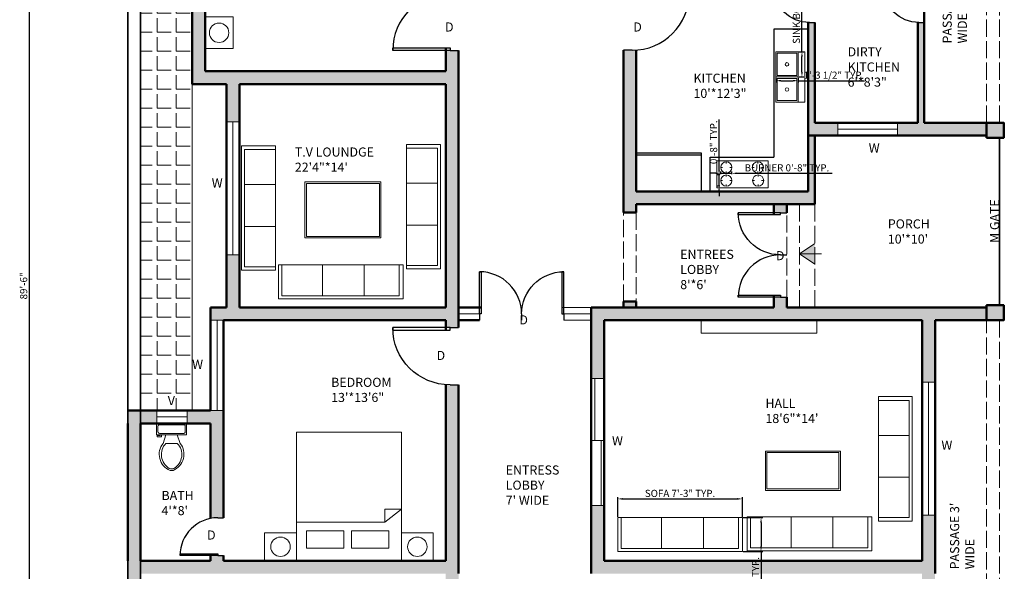
# Model space of a CAD drawing. Units: inches. Extents: x 554 to 1300, y 1707 to 2873.
# Tile 2 of 3: x 554 to 1242, y 2105 to 2490. Entities that reach past the tile are written whole.
import ezdxf

# ---------------------------------------------------------------- set-up
doc = ezdxf.new("R2010")
doc.units = ezdxf.units.IN
doc.linetypes.add('ACAD_ISO02W100', pattern=[15, 12, -3])
for name, color, linetype, lineweight in [('A-ANNO-DIMS', 145, 'Continuous', 18), ('A-ANNO-PATT', 7, 'Continuous', 13), ('A-ANNO-SYMB', 7, 'Continuous', 18), ('A-AREA-IDEN', 145, 'Continuous', 25), ('A-CASE', 8, 'Continuous', 25), ('A-EQPM', 9, 'Continuous', 18), ('A-FLOR-FIXT', 9, 'Continuous', 18), ('A-FLOR-OVHD', 8, 'ACAD_ISO02W100', 18), ('A-WALL-OVHD', 30, 'ACAD_ISO02W100', 18), ('A-WALL-PATT', 30, 'Continuous', 13), ('C-PROP', 30, 'Continuous', 35), ('C-PROP-OVHD', 30, 'ACAD_ISO02W100', 18), ('C-PVMT', 8, 'Continuous', 18), ('C-PVMT-PATT', 116, 'Continuous', 13), ('COLUMN', 30, 'Continuous', 50), ('DOOR', 52, 'Continuous', 25), ('FUR', 210, 'Continuous', 18), ('TEXT', 145, 'Continuous', 18), ('WALL', 30, 'Continuous', 50), ('WIND', 70, 'Continuous', 18)]:
    doc.layers.add(name, color=color, linetype=linetype, lineweight=lineweight)
doc.styles.get("Standard").update_dxf_attribs({"font": 'arial.ttf'})
doc.dimstyles.new('ISO-25', dxfattribs={"dimtxt": 5, "dimasz": 3.5, "dimexe": 1.25, "dimexo": 0.625, "dimtad": 1, "dimdec": 0, "dimlunit": 4, "dimtxsty": 'Standard', "dimcen": 2.5, "dimadec": 0, "dimazin": 0, "dimtfac": 1, "dimtdec": 0, "dimtmove": 0, "dimatfit": 3, "dimfxl": 1, "dimarcsym": 0})

# ---------------------------------------------------------------- blocks, each defined once
blk = doc.blocks.new('*U2')
for p, q in [((0, 0), (0, -6)), ((40, 0), (40, -6))]:
    blk.add_line(p, q)
blk.add_lwpolyline([(0, 0), (0, 40), (1.75, 40), (1.75, 0)], close=True)
blk.add_arc((0, 0), 40, 0, 90)
blk = doc.blocks.new('*U4')
for p, q in [((9.5, -6), (9.5, -2)), ((-10, -8.5), (-8, -8.5)), ((-10, -9.5), (-10, -8.5)), ((-7, -9.5), (-10, -9.5)), ((-8, -8.5), (-8, -8)), ((-7, -8), (-7, -9.5)), ((-4, -8), (-6, -14)), ((4, -8), (6, -14)), ((4, -14), (-4, -14))]:
    blk.add_line(p, q)
blk.add_lwpolyline([(10.5, -8), (10.5, 0), (-10.5, 0), (-10.5, -8)], close=True)
for points in [[(-9.5, -2), (-9.5, -6)], [(8.5, -1), (-8.5, -1)], [(-8.5, -7), (8.5, -7)]]:
    blk.add_lwpolyline(points)
for centre, radius, start, end in [((-8.62, -1.88), 0.884, 81.8699, 188.1301), ((-8.62, -6.12), 0.884, 171.8699, 278.1301), ((8.62, -1.88), 0.884, 351.8699, 98.1301), ((8.62, -6.12), 0.884, 261.8699, 8.1301), ((3.52, -21.58), 12.17, 141.46911, 247.97143), ((4.2, -21.82), 11.33, 136.36773, 238.94682), ((-3.52, -21.58), 12.17, 292.02843, 38.53071), ((-4.2, -21.82), 11.33, 301.05301, 43.63209), ((0, -27.88), 4, 245.73182, 294.26817), ((0, -29), 4, 254.86053, 285.13947)]:
    blk.add_arc(centre, radius, start, end)
blk = doc.blocks.new('*D8')
at = {"layer": 'A-ANNO-DIMS', "color": 0, "lineweight": -2, "transparency": 16777216}
for p, q in [((629.06, 2841.48), (559.64, 2841.48)), ((560.89, 2837.98), (560.89, 1770.98)), ((629.06, 1767.48), (559.64, 1767.48))]:
    blk.add_line(p, q, dxfattribs=at)
at = {"layer": 'A-ANNO-DIMS', "color": 0, "lineweight": 100, "transparency": 16777216}
for points in [[(560.3, 2837.98), (561.47, 2837.98), (560.89, 2841.48)], [(560.3, 1770.98), (561.47, 1770.98), (560.89, 1767.48)]]:
    blk.add_solid(points, dxfattribs=at)
at = {"layer": 'Defpoints', "color": 0, "lineweight": 100, "transparency": 16777216}
for p in [(629.68, 2841.48), (560.89, 1767.48), (629.68, 1767.48)]:
    blk.add_point(p, dxfattribs=at)
at = {"layer": 'A-ANNO-DIMS', "color": 0, "transparency": 16777216, "insert": (557.71, 2304.48), "char_height": 5, "attachment_point": 5, "rotation": 90}
blk.add_mtext('89\'-6"', dxfattribs=at)
blk = doc.blocks.new('SOFA-3SEAT')
for p, q in [((0, 84.31), (0, 87)), ((0, 87), (23.69, 87)), ((23.69, 87), (23.69, 0)), ((0, 59.83), (21.61, 59.83)), ((0, 30.66), (21.61, 30.66)), ((0, 0), (0, 5.47)), ((23.69, 0), (0, 0))]:
    blk.add_line(p, q)
blk.add_lwpolyline([(21.61, 84.31), (0, 84.31), (0, 2.38), (21.61, 2.38)], close=True)
blk = doc.blocks.new('NIGHTSTAND')
blk.add_lwpolyline([(22.14, 19.58), (0, 19.58), (0, 0), (22.14, 0)], close=True)
blk.add_circle((11.07, 9.79), 6.79)
blk = doc.blocks.new('TABLE-COFFEE')
for points in [[(52.29, 0), (0, 0), (0, 27.46), (52.29, 27.46)], [(51.29, 1), (1, 1), (1, 26.46), (51.29, 26.46)]]:
    blk.add_lwpolyline(points, close=True)
blk = doc.blocks.new('COOKTOP-BURNER')
for p, q in [((3.89, 7.77), (3.89, 6.66)), ((0, 3.89), (1.24, 3.89)), ((3.89, 0), (3.89, 1.05)), ((7.77, 3.89), (6.32, 3.89))]:
    blk.add_line(p, q)
blk.add_circle((3.89, 3.89), 3.89)
blk = doc.blocks.new('SINK-BOWL-RECT')
for points in [[(0, 0), (15.58, 0), (15.58, 17.58), (0, 17.58)], [(1, 1), (14.58, 1), (14.58, 16.58), (1, 16.58)]]:
    blk.add_lwpolyline(points, close=True)
blk.add_circle((7.79, 8.79), 1.21)
blk = doc.blocks.new('*D16')
at = {"layer": 'A-ANNO-DIMS', "color": 0, "lineweight": -2, "transparency": 16777216}
for p, q in [((971.7, 2143.27), (971.7, 2156.95)), ((975.2, 2155.7), (1055.2, 2155.7)), ((1058.7, 2143.27), (1058.7, 2156.95))]:
    blk.add_line(p, q, dxfattribs=at)
at = {"layer": 'A-ANNO-DIMS', "color": 0, "lineweight": 100, "transparency": 16777216}
for points in [[(975.2, 2156.28), (975.2, 2155.11), (971.7, 2155.7)], [(1055.2, 2156.28), (1055.2, 2155.11), (1058.7, 2155.7)]]:
    blk.add_solid(points, dxfattribs=at)
at = {"layer": 'Defpoints', "color": 0, "lineweight": 100, "transparency": 16777216}
for p in [(1058.7, 2155.7), (971.7, 2142.65), (1058.7, 2142.65)]:
    blk.add_point(p, dxfattribs=at)
at = {"layer": 'A-ANNO-DIMS', "color": 0, "transparency": 16777216, "insert": (1015.2, 2158.91), "char_height": 5, "attachment_point": 5}
blk.add_mtext('SOFA 7\'-3" TYP.', dxfattribs=at)
blk = doc.blocks.new('*D17')
at = {"layer": 'A-ANNO-DIMS', "color": 0, "lineweight": -2, "transparency": 16777216}
for p, q in [((1059.32, 2142.65), (1073, 2142.65)), ((1071.75, 2139.15), (1071.75, 2122.46)), ((1059.32, 2118.96), (1073, 2118.96)), ((1071.75, 2118.96), (1071.75, 2068.67))]:
    blk.add_line(p, q, dxfattribs=at)
at = {"layer": 'A-ANNO-DIMS', "color": 0, "lineweight": 100, "transparency": 16777216}
for points in [[(1071.16, 2139.15), (1072.33, 2139.15), (1071.75, 2142.65)], [(1071.16, 2122.46), (1072.33, 2122.46), (1071.75, 2118.96)]]:
    blk.add_solid(points, dxfattribs=at)
at = {"layer": 'Defpoints', "color": 0, "lineweight": 100, "transparency": 16777216}
for p in [(1058.7, 2142.65), (1058.7, 2118.96), (1071.75, 2118.96)]:
    blk.add_point(p, dxfattribs=at)
at = {"layer": 'A-ANNO-DIMS', "color": 0, "transparency": 16777216, "insert": (1068.54, 2092.06), "char_height": 5, "attachment_point": 5, "rotation": 90}
blk.add_mtext('1\'-11 1/2" TYP.', dxfattribs=at)
blk = doc.blocks.new('*D20')
at = {"layer": 'A-ANNO-DIMS', "color": 0, "lineweight": -2, "transparency": 16777216}
for p, q in [((1040.11, 2383.13), (1036.61, 2383.13)), ((1043.61, 2382.59), (1043.61, 2384.38)), ((1043.61, 2383.13), (1051.38, 2383.13)), ((1051.38, 2382.59), (1051.38, 2384.38)), ((1054.88, 2383.13), (1121.32, 2383.13))]:
    blk.add_line(p, q, dxfattribs=at)
at = {"layer": 'A-ANNO-DIMS', "color": 0, "lineweight": 100, "transparency": 16777216}
for points in [[(1040.11, 2383.71), (1040.11, 2382.54), (1043.61, 2383.13)], [(1054.88, 2383.71), (1054.88, 2382.54), (1051.38, 2383.13)]]:
    blk.add_solid(points, dxfattribs=at)
at = {"layer": 'Defpoints', "color": 0, "lineweight": 100, "transparency": 16777216}
for p in [(1043.61, 2381.96), (1051.38, 2383.13), (1051.38, 2381.96)]:
    blk.add_point(p, dxfattribs=at)
at = {"layer": 'A-ANNO-DIMS', "color": 0, "transparency": 16777216, "insert": (1089.85, 2386.31), "char_height": 5, "attachment_point": 5}
blk.add_mtext('BURNER 0\'-8" TYP.', dxfattribs=at)
blk = doc.blocks.new('*D21')
at = {"layer": 'A-ANNO-DIMS', "color": 0, "lineweight": -2, "transparency": 16777216}
for p, q in [((1042.44, 2385.46), (1042.44, 2420.69)), ((1042.98, 2381.96), (1041.19, 2381.96)), ((1042.44, 2374.19), (1042.44, 2381.96)), ((1042.98, 2374.19), (1041.19, 2374.19)), ((1042.44, 2370.69), (1042.44, 2367.19))]:
    blk.add_line(p, q, dxfattribs=at)
at = {"layer": 'A-ANNO-DIMS', "color": 0, "lineweight": 100, "transparency": 16777216}
for points in [[(1041.86, 2385.46), (1043.02, 2385.46), (1042.44, 2381.96)], [(1041.86, 2370.69), (1043.02, 2370.69), (1042.44, 2374.19)]]:
    blk.add_solid(points, dxfattribs=at)
at = {"layer": 'Defpoints', "color": 0, "lineweight": 100, "transparency": 16777216}
for p in [(1042.44, 2381.96), (1043.61, 2381.96), (1043.61, 2374.19)]:
    blk.add_point(p, dxfattribs=at)
at = {"layer": 'A-ANNO-DIMS', "color": 0, "transparency": 16777216, "insert": (1039.26, 2404.83), "char_height": 5, "attachment_point": 5, "rotation": 90}
blk.add_mtext('0\'-8" TYP.', dxfattribs=at)
blk = doc.blocks.new('*D28')
at = {"layer": 'A-ANNO-DIMS', "color": 0, "lineweight": -2, "transparency": 16777216}
for p, q in [((1100.29, 2468.04), (1100.29, 2555.65)), ((1098.27, 2468.04), (1101.54, 2468.04)), ((1100.29, 2453.96), (1100.29, 2464.54)), ((1098.27, 2450.46), (1101.54, 2450.46))]:
    blk.add_line(p, q, dxfattribs=at)
at = {"layer": 'A-ANNO-DIMS', "color": 0, "lineweight": 100, "transparency": 16777216}
for points in [[(1099.7, 2464.54), (1100.87, 2464.54), (1100.29, 2468.04)], [(1099.7, 2453.96), (1100.87, 2453.96), (1100.29, 2450.46)]]:
    blk.add_solid(points, dxfattribs=at)
at = {"layer": 'Defpoints', "color": 0, "lineweight": 100, "transparency": 16777216}
for p in [(1097.65, 2468.04), (1100.29, 2468.04), (1097.65, 2450.46)]:
    blk.add_point(p, dxfattribs=at)
at = {"layer": 'A-ANNO-DIMS', "color": 0, "transparency": 16777216, "insert": (1097.07, 2513.59), "char_height": 5, "attachment_point": 5, "rotation": 90}
blk.add_mtext('SINK BOWL 1\'-5 1/2" TYP.', dxfattribs=at)
blk = doc.blocks.new('*D29')
at = {"layer": 'A-ANNO-DIMS', "color": 0, "lineweight": -2, "transparency": 16777216}
for p, q in [((1082.07, 2449.84), (1082.07, 2446.58)), ((1085.57, 2447.83), (1094.15, 2447.83)), ((1097.65, 2449.84), (1097.65, 2446.58)), ((1097.65, 2447.83), (1144.06, 2447.83))]:
    blk.add_line(p, q, dxfattribs=at)
at = {"layer": 'A-ANNO-DIMS', "color": 0, "lineweight": 100, "transparency": 16777216}
for points in [[(1085.57, 2448.41), (1085.57, 2447.24), (1082.07, 2447.83)], [(1094.15, 2448.41), (1094.15, 2447.24), (1097.65, 2447.83)]]:
    blk.add_solid(points, dxfattribs=at)
at = {"layer": 'Defpoints', "color": 0, "lineweight": 100, "transparency": 16777216}
for p in [(1082.07, 2450.46), (1097.65, 2450.46), (1097.65, 2447.83)]:
    blk.add_point(p, dxfattribs=at)
at = {"layer": 'A-ANNO-DIMS', "color": 0, "transparency": 16777216, "insert": (1122.6, 2451.04), "char_height": 5, "attachment_point": 5}
blk.add_mtext('1\'-3 1/2" TYP.', dxfattribs=at)

msp = doc.modelspace()

# ---------------------------------------------------------------- hatches: boundary and pattern name
at = {"layer": 'A-ANNO-PATT'}
h = msp.add_hatch(color=256, dxfattribs=at)
h.dxf.hatch_style = 1
h.paths.add_polyline_path([(1109.18, 2334.01), (1098.6, 2326.82), (1109.18, 2326.82)])
h.paths.add_polyline_path([(1109.18, 2326.82), (1098.6, 2326.82), (1109.18, 2319.63)])
at = {"layer": 'A-WALL-PATT'}
h = msp.add_hatch(color=256, dxfattribs=at)
h.dxf.hatch_style = 1
h.paths.add_polyline_path([(1136.18, 2067.48), (1026.18, 2067.48), (1026.18, 2065.48), (1134.18, 2065.48), (1134.18, 2039.48), (1026.18, 2039.48), (1026.18, 2037.48), (1136.18, 2037.48)])
h.paths.add_polyline_path([(1193.18, 2103.48), (1184.18, 2103.48), (1184.18, 2077.52), (1193.18, 2077.52)])
h.paths.add_polyline_path([(1193.18, 2032.94), (1184.18, 2032.94), (1184.18, 2001.48), (1148.18, 2001.48), (1136.18, 2001.48), (1128.74, 2001.48), (1128.74, 1992.48), (1193.18, 1992.48), (1193.18, 2001.48)])
h.paths.add_polyline_path([(1076.18, 2001.48), (1045.59, 2001.48), (1045.59, 1992.48), (1076.18, 1992.48)])
h.paths.add_polyline_path([(993.02, 2001.48), (923.53, 2001.48), (923.53, 1996.9), (923.53, 1992.48), (993.02, 1992.48)])
h.paths.add_polyline_path([(1184.18, 2112.48), (962.18, 2112.48), (962.18, 2151.15), (953.18, 2151.15), (953.18, 2103.48), (1184.18, 2103.48)])
h.paths.add_polyline_path([(1193.18, 2144.33), (1184.18, 2144.33), (1184.18, 2112.48), (1184.18, 2103.48), (1193.18, 2103.48)])
h.paths.add_polyline_path([(772.18, 2796.48), (758.22, 2796.48), (758.22, 2787.48), (767.68, 2787.48), (772.18, 2787.48)])
h.paths.add_polyline_path([(737.06, 2796.48), (674.68, 2796.48), (674.68, 2710.98), (683.68, 2710.98), (683.68, 2715.48), (683.68, 2787.48), (737.06, 2787.48)])
h.paths.add_polyline_path([(786.15, 2796.48), (772.18, 2796.48), (772.18, 2787.48), (786.15, 2787.48)])
h.paths.add_polyline_path([(860.68, 2796.48), (807.31, 2796.48), (807.31, 2787.48), (856.18, 2787.48), (860.68, 2787.48)])
h.paths.add_polyline_path([(905.53, 2796.48), (860.68, 2796.48), (860.68, 2787.48), (905.53, 2787.48)])
h.paths.add_polyline_path([(860.68, 2787.48), (856.18, 2787.48), (856.18, 2715.48), (853.67, 2715.48), (853.67, 2713.96), (853.67, 2710.98), (856.18, 2710.98), (860.68, 2710.98)])
h.paths.add_polyline_path([(772.18, 2787.48), (767.68, 2787.48), (767.68, 2715.48), (728.12, 2715.48), (706.98, 2715.48, -0.019152), (707.04, 2713.96), (707.04, 2710.98), (772.18, 2710.98)])
h.paths.add_polyline_path([(833.86, 2715.48), (772.18, 2715.48), (772.18, 2710.98), (833.8, 2710.98), (833.8, 2713.96, -0.019152)])
h.paths.add_polyline_path([(1025.68, 2796.48), (981.39, 2796.48), (981.39, 2787.48), (1001.03, 2787.48), (1016.68, 2787.48), (1025.68, 2787.48)])
h.paths.add_polyline_path([(1094.68, 2796.48), (1025.68, 2796.48), (1025.68, 2787.48), (1085.68, 2787.48), (1094.68, 2787.48)])
h.paths.add_polyline_path([(1140.18, 2796.48), (1094.68, 2796.48), (1094.68, 2787.48), (1140.18, 2787.48)], flags=17)
h.paths.add_polyline_path([(1185.68, 2796.48), (1161.35, 2796.48), (1161.35, 2787.48), (1176.68, 2787.48), (1176.68, 2736.68), (1176.72, 2736.68), (1176.72, 2715.48), (1137.16, 2715.48), (1094.68, 2715.48), (1094.68, 2706.48), (1185.68, 2706.48)])
h.paths.add_polyline_path([(1094.68, 2787.48), (1085.68, 2787.48), (1085.68, 2748.92), (1090.01, 2748.92, -0.040642), (1094.68, 2748.54)])
h.paths.add_polyline_path([(1025.68, 2787.48), (1016.68, 2787.48), (1016.68, 2607.48), (1016.68, 2598.48), (1025.68, 2598.48), (1025.68, 2672.36), (1025.68, 2706.48)])
h.paths.add_polyline_path([(1094.68, 2715.48), (1094.68, 2720.05), (1090.01, 2720.05), (1085.68, 2720.05), (1085.68, 2715.48), (1082.66, 2715.48), (1082.66, 2706.48), (1094.68, 2706.48)])
h.paths.add_polyline_path([(1043.78, 2715.48), (1025.68, 2715.48), (1025.68, 2706.48), (1043.78, 2706.48)])
h.paths.add_polyline_path([(1185.68, 2577.7), (1176.68, 2577.7), (1176.68, 2570), (1176.68, 2526.48), (1176.68, 2517.48), (1185.68, 2517.48)])
h.paths.add_polyline_path([(1185.68, 2706.48), (1176.68, 2706.48), (1176.68, 2670.52), (1185.68, 2670.52)])
h.paths.add_polyline_path([(1025.68, 2598.48), (1016.68, 2598.48), (1016.68, 2569.99), (1022.68, 2569.99, -0.01877), (1025.68, 2569.88)])
h.paths.add_polyline_path([(1016.68, 2607.48), (903.83, 2607.48, -0.01877), (903.94, 2604.48), (903.94, 2598.48), (1016.68, 2598.48)])
h.paths.add_polyline_path([(860.68, 2646.48), (851.68, 2646.48), (851.68, 2508.85, -0.01877), (854.68, 2508.96), (860.68, 2508.96)])
h.paths.add_polyline_path([(863.94, 2604.48), (863.94, 2607.48), (860.68, 2607.48), (860.68, 2598.48), (863.94, 2598.48)])
h.paths.add_polyline_path([(1101.44, 2750.41), (1134.65, 2750.41), (1134.65, 2774.1), (1101.44, 2774.1)], flags=25)
h.paths.add_polyline_path([(1049.21, 2750.31), (1082.94, 2750.31), (1082.94, 2773.99), (1049.21, 2773.99)], flags=9)
h = msp.add_hatch(color=256, dxfattribs=at)
h.dxf.hatch_style = 1
h.paths.add_polyline_path([(683.68, 2710.98), (674.68, 2710.98), (674.68, 2646.48), (674.68, 2589.67), (683.68, 2589.67), (683.68, 2646.48), (683.68, 2650.98)])
h.paths.add_polyline_path([(688.17, 2650.98), (683.68, 2650.98), (683.68, 2646.48), (688.17, 2646.48)])
h.paths.add_polyline_path([(772.18, 2710.98), (767.68, 2710.98), (767.68, 2650.98), (730.85, 2650.98), (730.85, 2646.48), (772.18, 2646.48)])
h.paths.add_polyline_path([(860.68, 2710.98), (856.18, 2710.98), (856.18, 2650.98), (772.18, 2650.98), (772.18, 2646.48), (860.68, 2646.48)])
h.paths.add_polyline_path([(683.68, 2496.84), (674.68, 2496.84), (674.68, 2445.48), (683.68, 2445.48), (683.68, 2454.48)])
h.paths.add_polyline_path([(851.68, 2454.48), (683.68, 2454.48), (683.68, 2445.48), (851.68, 2445.48)])
h.paths.add_polyline_path([(707.68, 2445.48), (698.68, 2445.48), (698.68, 2419.1), (707.68, 2419.1)])
h.paths.add_polyline_path([(698.68, 2289.48), (687.57, 2289.48), (687.57, 2280.48), (696.57, 2280.48), (698.68, 2280.48)])
h.paths.add_polyline_path([(687.57, 2217.48), (671.17, 2217.48), (671.17, 2208.48), (687.57, 2208.48)])
h.paths.add_polyline_path([(650.01, 2217.48), (638.68, 2217.48), (638.68, 2208.48), (650.01, 2208.48)])
h.paths.add_polyline_path([(860.68, 2235.34), (854.68, 2235.34, -0.01877), (851.68, 2235.45), (851.68, 2112.48), (696.57, 2112.48), (696.57, 2103.48), (860.68, 2103.48)])
h.paths.add_polyline_path([(666.88, 1959.48), (647.68, 1959.48), (638.68, 1959.48), (638.68, 1950.48), (647.68, 1950.48), (666.88, 1950.48)])
h.paths.add_polyline_path([(756.66, 1959.48), (719.44, 1959.48), (719.44, 1950.48), (756.66, 1950.48)])
h.paths.add_polyline_path([(860.68, 1992.48), (864.62, 1992.48), (864.62, 1996.9), (864.62, 2001.48), (860.68, 2001.48), (860.68, 2058.13), (854.68, 2058.13, -0.01877), (851.68, 2058.24), (851.68, 1992.48), (851.68, 1959.48), (809.22, 1959.48), (809.22, 1950.48), (860.68, 1950.48)])
h.paths.add_polyline_path([(860.68, 2103.48), (851.68, 2103.48), (851.68, 2098.13), (854.68, 2098.13), (860.68, 2098.13)])
h.paths.add_polyline_path([(984.68, 2397.2), (984.68, 2469.19, -0.01877), (981.68, 2469.08), (975.68, 2469.08), (975.68, 2361.48), (975.68, 2355.65), (984.68, 2355.65), (984.68, 2361.48), (984.68, 2370.48)])
h.paths.add_polyline_path([(1109.18, 2409.48), (1104.68, 2409.48), (1104.68, 2370.48), (984.68, 2370.48), (984.68, 2361.48), (1109.18, 2361.48)])
h.paths.add_polyline_path([(1125.26, 2418.48), (1109.18, 2418.48), (1109.18, 2488.51), (1105.47, 2488.51, -0.008003), (1104.68, 2488.52), (1104.68, 2409.48), (1109.18, 2409.48), (1125.26, 2409.48)])
h.paths.add_polyline_path([(1185.68, 2418.48), (1167, 2418.48), (1167, 2409.48), (1185.68, 2409.48)])
h.paths.add_polyline_path([(1185.68, 2488.51), (1181.97, 2488.51, -0.008003), (1181.18, 2488.52), (1181.18, 2418.48), (1185.68, 2418.48)])
h.paths.add_polyline_path([(1025.68, 2529.99), (1022.68, 2529.99), (1016.68, 2529.99), (1016.68, 2526.48), (975.68, 2526.48), (975.68, 2517.48), (1025.68, 2517.48)])
h.paths.add_polyline_path([(984.68, 2517.48), (975.68, 2517.48), (975.68, 2509.08), (981.68, 2509.08), (984.68, 2509.08)])
h.paths.add_polyline_path([(1176.68, 2526.48), (1025.68, 2526.48), (1025.68, 2517.48), (1104.68, 2517.48), (1176.68, 2517.48)])
h.paths.add_polyline_path([(745.17, 1864.25), (773.96, 1864.25), (773.96, 1877.33), (745.17, 1877.33)], flags=9)
h = msp.add_hatch(color=256, dxfattribs=at)
h.dxf.hatch_style = 1
h.paths.add_polyline_path([(638.68, 2072.33), (638.68, 2103.48), (638.68, 2217.48), (629.68, 2217.48), (629.68, 2097.48), (629.68, 1992.48), (629.68, 1950.48), (638.68, 1950.48), (638.68, 1992.48)])
h.paths.add_polyline_path([(696.57, 2217.48), (687.57, 2217.48), (687.57, 2142.07, -0.048021), (692.61, 2142.55), (696.57, 2142.55)])
h.paths.add_polyline_path([(696.57, 2116.14), (692.61, 2116.14), (687.57, 2116.14), (687.57, 2112.48), (638.68, 2112.48), (638.68, 2103.48), (687.57, 2103.48), (696.57, 2103.48), (696.57, 2112.48)])
h.paths.add_polyline_path([(1010.14, 2078.06), (1025.63, 2078.06), (1025.63, 2091.14), (1010.14, 2091.14)], flags=9)
h.paths.add_polyline_path([(1129.91, 2440.07), (1172.04, 2440.07), (1172.04, 2474.45), (1129.91, 2474.45)], flags=9)
h.paths.add_polyline_path([(1022.04, 2432.2), (1064.45, 2432.2), (1064.45, 2455.89), (1022.04, 2455.89)], flags=9)
h.paths.add_polyline_path([(891.25, 2147.87), (936.31, 2147.87), (936.31, 2182.23), (891.25, 2182.23)], flags=9)
h.paths.add_polyline_path([(951.1, 2040.21), (1005.03, 2040.21), (1005.03, 2063.9), (951.1, 2063.9)], flags=9)
h.paths.add_polyline_path([(988, 1912.76), (1023.48, 1912.76), (1023.48, 1936.45), (988, 1936.45)], flags=9)
h.paths.add_polyline_path([(735.06, 2044.01), (781.37, 2044.01), (781.37, 2078.39), (735.06, 2078.39)], flags=9)
h.paths.add_polyline_path([(651.07, 2140.85), (677.89, 2140.85), (677.89, 2164.54), (651.07, 2164.54)], flags=9)
h.paths.add_polyline_path([(769.16, 2219.79), (818.47, 2219.79), (818.47, 2243.48), (769.16, 2243.48)], flags=9)
h.paths.add_polyline_path([(745.28, 2587.79), (794.59, 2587.79), (794.59, 2611.48), (745.28, 2611.48)], flags=9)
h = msp.add_hatch(color=256, dxfattribs=at)
h.dxf.hatch_style = 1
h.paths.add_polyline_path([(994.52, 1776.48), (982.92, 1776.48), (982.92, 1765.92), (994.52, 1765.92)])
h.paths.add_polyline_path([(1044.88, 1776.48), (1033.28, 1776.48), (1033.28, 1765.92), (1044.88, 1765.92)])
h.paths.add_polyline_path([(1226.37, 1776.48), (1214.77, 1776.48), (1214.77, 1765.92), (1226.37, 1765.92)])
h.paths.add_polyline_path([(1241.1, 2418.48), (1229.18, 2418.48), (1229.18, 2407.99), (1241.1, 2407.99)])
h.paths.add_polyline_path([(1241.1, 2290.97), (1229.18, 2290.97), (1229.18, 2280.48), (1238.18, 2280.48), (1241.1, 2280.48)])
h.paths.add_polyline_path([(1229.18, 2418.48), (1185.68, 2418.48), (1185.68, 2409.48), (1229.18, 2409.48)])
h.paths.add_polyline_path([(1229.18, 2289.48), (1089.68, 2289.48), (1089.68, 2280.48), (1110.8, 2280.48), (1184.18, 2280.48), (1193.18, 2280.48), (1229.18, 2280.48)])
h.paths.add_polyline_path([(1193.18, 2280.48), (1184.18, 2280.48), (1184.18, 2237.16), (1193.18, 2237.16)])
h.paths.add_polyline_path([(1089.68, 2289.48), (953.18, 2289.48), (953.18, 2280.48), (953.18, 2239.7), (962.18, 2239.7), (962.18, 2280.48), (1089.68, 2280.48)])
h.paths.add_polyline_path([(860.68, 2289.48), (851.68, 2289.48), (851.68, 2280.48), (860.68, 2280.48)])
h.paths.add_polyline_path([(860.68, 2280.48), (851.68, 2280.48), (851.68, 2275.34), (854.68, 2275.34), (860.68, 2275.34)])
h.paths.add_polyline_path([(860.68, 2445.48), (860.68, 2468.96), (854.68, 2468.96), (851.68, 2468.96), (851.68, 2454.48), (851.68, 2445.48), (851.68, 2289.48), (860.68, 2289.48)])
h.paths.add_polyline_path([(851.68, 2289.48), (707.68, 2289.48), (707.68, 2326.28), (698.68, 2326.28), (698.68, 2280.48), (851.68, 2280.48)])
h.paths.add_polyline_path([(1241.54, 2332.25), (1241.54, 2369.42), (1228.46, 2369.42), (1228.46, 2332.25)], flags=9)
h.paths.add_polyline_path([(1157.71, 2330.44), (1193.19, 2330.44), (1193.19, 2354.12), (1157.71, 2354.12)], flags=9)
h = msp.add_hatch(color=256, dxfattribs=at)
h.dxf.hatch_style = 1
h.paths.add_polyline_path([(1089.68, 2361.48), (1080.68, 2361.48), (1080.68, 2355.61), (1085.26, 2355.61), (1089.68, 2355.61)])
h.paths.add_polyline_path([(1089.68, 2296.71), (1085.26, 2296.71), (1080.68, 2296.71), (1080.68, 2289.48), (1089.68, 2289.48)])
h = msp.add_hatch(color=256, dxfattribs=at)
h.dxf.hatch_style = 1
h.paths.add_polyline_path([(984.68, 2293.56), (975.68, 2293.56), (975.68, 2289.48), (984.68, 2289.48)])
at = {"layer": 'C-PVMT-PATT'}
h = msp.add_hatch(dxfattribs=at)
h.set_pattern_fill('ANGLE', color=256, scale=1.9)
h.set_pattern_definition([(0, (0, 0), (0, 13.2715), [9.652, -3.6195]), (90, (0, 0), (-13.2715, 8e-16), [9.652, -3.6195])])
h.paths.add_polyline_path([(674.68, 2646.48), (674.68, 2710.98), (674.68, 2796.48), (772.18, 2796.48), (860.68, 2796.48), (1025.68, 2796.48), (1025.68, 2832.48), (638.68, 2832.48), (638.68, 2217.48), (674.68, 2217.48), (674.68, 2445.48)])

# ---------------------------------------------------------------- linework, layer by layer
at = {"layer": 'A-ANNO-SYMB'}
for p, q in [((1098.6, 2326.82), (1109.18, 2334.01)), ((1114.02, 2326.82), (1098.6, 2326.82)), ((1098.6, 2326.82), (1109.18, 2319.63))]:
    msp.add_line(p, q, dxfattribs=at)
at = {"layer": 'A-CASE'}
for p, q in [((1104.68, 2483.8), (1080.68, 2483.8)), ((1080.68, 2483.8), (1080.68, 2394.48)), ((1030.18, 2395.87), (984.68, 2395.87)), ((1036.23, 2370.48), (1036.23, 2394.48)), ((1036.23, 2394.48), (1080.68, 2394.48))]:
    msp.add_line(p, q, dxfattribs=at)
msp.add_lwpolyline([(984.68, 2370.48), (1030.18, 2370.48), (1030.18, 2397.2), (984.68, 2397.2)], close=True, dxfattribs=at)
at = {"layer": 'A-EQPM'}
msp.add_lwpolyline([(1040.83, 2391.82), (1076.83, 2391.82), (1076.83, 2372.88), (1040.83, 2372.88)], close=True, dxfattribs=at)
at = {"layer": 'A-FLOR-FIXT'}
for p, q in [((1097.65, 2468.04), (1097.65, 2432.89)), ((1082.07, 2450.46), (1097.65, 2450.46))]:
    msp.add_line(p, q, dxfattribs=at)
msp.add_lwpolyline([(1082.07, 2432.89), (1102.31, 2432.89), (1102.31, 2468.04), (1082.07, 2468.04)], close=True, dxfattribs=at)
at = {"layer": 'A-FLOR-OVHD'}
for p, q in [((1098.6, 2361.48), (1098.6, 2289.48)), ((1109.18, 2361.48), (1109.18, 2289.48)), ((1089.68, 2296.71), (1089.68, 2355.61))]:
    msp.add_line(p, q, dxfattribs=at)
at = {"layer": 'A-WALL-OVHD'}
msp.add_lwpolyline([(975.68, 2355.65), (984.68, 2355.65), (984.68, 2293.56), (975.68, 2293.56)], close=True, dxfattribs=at)
at = {"layer": 'C-PROP'}
for p, q in [((629.68, 2841.48), (629.68, 2097.48)), ((638.68, 2832.48), (638.68, 2097.48)), ((1238.18, 2407.99), (1238.18, 2290.97))]:
    msp.add_line(p, q, dxfattribs=at)
at = {"layer": 'C-PROP-OVHD'}
for points in [[(1229.18, 2418.48), (1238.18, 2418.48), (1238.18, 2670.52), (1229.18, 2670.52)], [(1238.18, 2001.48), (1229.18, 2001.48), (1229.18, 2280.48), (1238.18, 2280.48)]]:
    msp.add_lwpolyline(points, close=True, dxfattribs=at)
at = {"layer": 'C-PVMT'}
msp.add_line((674.68, 2445.48), (674.68, 2217.48), dxfattribs=at)
at = {"layer": 'COLUMN'}
msp.add_lwpolyline([(1229.18, 2407.99), (1241.1, 2407.99), (1241.1, 2418.48), (1229.18, 2418.48)], close=True, dxfattribs=at)
msp.add_lwpolyline([(1229.18, 2280.48), (1241.1, 2280.48), (1241.1, 2290.97), (1229.18, 2290.97), (1229.18, 2289.48)], dxfattribs=at)
at = {"layer": 'FUR'}
for p, q in [((732.86, 2402.39), (709.17, 2402.39)), ((709.17, 2402.39), (709.17, 2315.39)), ((732.86, 2315.39), (732.86, 2402.39)), ((732.86, 2375.22), (711.24, 2375.22)), ((732.86, 2346.05), (711.24, 2346.05)), ((709.17, 2315.39), (732.86, 2315.39)), ((809.07, 2139.54), (809.07, 2148.53)), ((809.07, 2148.53), (820.77, 2148.53)), ((820.77, 2148.53), (809.07, 2139.54)), ((747.41, 2139.54), (809.07, 2139.54))]:
    msp.add_line(p, q, dxfattribs=at)
for points in [[(711.24, 2399.7), (732.86, 2399.7), (732.86, 2317.77), (711.24, 2317.77)], [(753.4, 2377.13), (806.47, 2377.13), (806.47, 2338.05), (753.4, 2338.05)], [(754.4, 2376.13), (805.47, 2376.13), (805.47, 2339.05), (754.4, 2339.05)], [(1029.95, 2271.55), (1110.8, 2271.55), (1110.8, 2280.48), (1029.95, 2280.48)], [(747.41, 2112.48), (820.77, 2112.48), (820.77, 2202.35), (747.41, 2202.35)], [(754.46, 2121.19), (780.52, 2121.19), (780.52, 2133.5), (754.46, 2133.5)], [(785.97, 2121.19), (812.04, 2121.19), (812.04, 2133.5), (785.97, 2133.5)]]:
    msp.add_lwpolyline(points, close=True, dxfattribs=at)
at = {"layer": 'WALL'}
for p, q in [((674.68, 2646.48), (674.68, 2445.48)), ((683.68, 2646.48), (683.68, 2454.48)), ((1185.68, 2517.48), (1185.68, 2418.48)), ((1104.68, 2409.48), (1104.68, 2488.52)), ((1109.18, 2418.48), (1109.18, 2488.51)), ((1181.18, 2488.52), (1181.18, 2418.48)), ((851.68, 2454.48), (851.68, 2470.71)), ((860.68, 2445.48), (860.68, 2468.96)), ((975.68, 2469.08), (975.68, 2361.48)), ((984.68, 2469.19), (984.68, 2370.48)), ((683.68, 2454.48), (851.68, 2454.48)), ((674.68, 2445.48), (698.68, 2445.48)), ((698.68, 2445.48), (698.68, 2289.48)), ((851.68, 2445.48), (707.68, 2445.48)), ((707.68, 2445.48), (707.68, 2289.48)), ((707.68, 2445.48), (851.68, 2445.48)), ((851.68, 2445.48), (851.68, 2289.48)), ((860.68, 2445.48), (860.68, 2280.48)), ((1181.18, 2418.48), (1109.18, 2418.48)), ((1109.18, 2418.48), (1181.18, 2418.48)), ((1185.68, 2418.48), (1238.18, 2418.48)), ((1229.18, 2409.48), (1229.18, 2418.48)), ((1185.68, 2409.48), (1104.68, 2409.48)), ((1104.68, 2370.48), (1104.68, 2409.48)), ((1109.18, 2361.48), (1109.18, 2409.48)), ((1109.18, 2409.48), (1229.18, 2409.48)), ((984.68, 2370.48), (1104.68, 2370.48)), ((975.68, 2361.48), (975.68, 2355.65)), ((984.68, 2361.48), (1109.18, 2361.48)), ((984.68, 2361.48), (984.68, 2355.65)), ((1080.68, 2354.32), (1080.68, 2361.48)), ((1089.68, 2355.61), (1089.68, 2361.48)), ((975.68, 2355.65), (984.68, 2355.65)), ((1080.68, 2289.48), (1080.68, 2297.99)), ((1089.68, 2289.48), (1089.68, 2296.71)), ((687.57, 2280.48), (687.57, 2289.48)), ((687.57, 2289.48), (698.68, 2289.48)), ((851.68, 2289.48), (707.68, 2289.48)), ((876.47, 2289.48), (860.68, 2289.48)), ((953.18, 2289.48), (953.18, 2103.48)), ((1080.68, 2289.48), (953.18, 2289.48)), ((975.68, 2293.56), (984.68, 2293.56)), ((975.68, 2293.56), (975.68, 2289.48)), ((984.68, 2293.56), (984.68, 2289.48)), ((984.68, 2289.48), (1080.68, 2289.48)), ((1229.18, 2289.48), (1089.68, 2289.48)), ((1184.18, 2289.48), (1089.68, 2289.48)), ((1229.18, 2289.48), (1229.18, 2280.48)), ((687.57, 2280.48), (687.57, 2217.48)), ((698.68, 2280.48), (696.57, 2280.48)), ((696.57, 2280.48), (696.57, 2142.55)), ((851.68, 2280.48), (698.68, 2280.48)), ((851.68, 2280.48), (797.18, 2280.48)), ((851.68, 2280.48), (851.68, 2273.59)), ((860.68, 2280.48), (860.68, 2275.34)), ((875.18, 2280.48), (860.68, 2280.48)), ((875.18, 2280.48), (860.68, 2280.48)), ((1184.18, 2280.48), (962.18, 2280.48)), ((962.18, 2280.48), (962.18, 2112.48)), ((1184.18, 2280.48), (971.18, 2280.48)), ((975.68, 2280.48), (1089.68, 2280.48)), ((1184.18, 2280.48), (1089.68, 2280.48)), ((1184.18, 2280.48), (1184.18, 2112.48)), ((1238.18, 2280.48), (1193.18, 2280.48)), ((1229.18, 2280.48), (1193.18, 2280.48)), ((1193.18, 2280.48), (1193.18, 2103.48)), ((1238.18, 2280.48), (1202.18, 2280.48)), ((851.68, 2235.45), (851.68, 2112.48)), ((860.68, 2235.34), (860.68, 2103.48)), ((638.68, 2217.48), (629.68, 2217.48)), ((638.68, 2217.48), (687.57, 2217.48)), ((629.68, 2112.48), (629.68, 2208.48)), ((638.68, 2208.48), (687.57, 2208.48)), ((638.68, 2112.48), (638.68, 2208.48)), ((687.57, 2208.48), (687.57, 2142.07)), ((687.57, 2117.29), (687.57, 2112.48)), ((687.57, 2112.48), (638.68, 2112.48)), ((696.57, 2116.14), (696.57, 2112.48)), ((851.68, 2112.48), (696.57, 2112.48)), ((962.18, 2112.48), (1184.18, 2112.48))]:
    msp.add_line(p, q, dxfattribs=at)
at = {"layer": 'WIND'}
for p, q in [((703.18, 2326.28), (703.18, 2419.1)), ((1125.26, 2413.98), (1167, 2413.98)), ((953.18, 2289.48), (932.8, 2289.48)), ((860.68, 2284.98), (875.18, 2284.9)), ((933.44, 2284.9), (953.18, 2284.9)), ((692.07, 2217.48), (692.07, 2280.48)), ((953.18, 2280.48), (934.09, 2280.48)), ((953.18, 2280.48), (934.09, 2280.48)), ((955.65, 2196.48), (955.65, 2239.7)), ((1188.68, 2144.33), (1188.68, 2237.16)), ((650.01, 2212.98), (671.17, 2212.98)), ((953.18, 2196.48), (962.18, 2196.48)), ((960.24, 2151.15), (960.24, 2196.48))]:
    msp.add_line(p, q, dxfattribs=at)
for points in [[(698.68, 2419.1), (707.68, 2419.1), (707.68, 2326.28), (698.68, 2326.28)], [(1125.26, 2418.48), (1167, 2418.48), (1167, 2409.48), (1125.26, 2409.48)], [(875.18, 2280.48), (860.68, 2280.48), (860.68, 2289.48), (875.18, 2289.48)], [(934.09, 2280.48), (953.18, 2280.48), (953.18, 2289.48), (934.09, 2289.48)], [(687.57, 2217.48), (696.57, 2217.48), (696.57, 2280.48), (687.57, 2280.48)], [(953.18, 2239.7), (962.18, 2239.7), (962.18, 2151.15), (953.18, 2151.15)], [(1184.18, 2237.16), (1193.18, 2237.16), (1193.18, 2144.33), (1184.18, 2144.33)], [(650.01, 2208.48), (671.17, 2208.48), (671.17, 2217.48), (650.01, 2217.48)]]:
    msp.add_lwpolyline(points, close=True, dxfattribs=at)

# ---------------------------------------------------------------- block references
at = {"layer": 'A-EQPM'}
for p in [(1043.61, 2383.34), (1065.63, 2383.34), (1043.61, 2374.19), (1065.83, 2374.19)]:
    msp.add_blockref('COOKTOP-BURNER', p, dxfattribs=at)
at = {"layer": 'A-FLOR-FIXT'}
for name, p in [('SINK-BOWL-RECT', (1082.07, 2450.46)), ('*U4', (660.33, 2208.48))]:
    msp.add_blockref(name, p, dxfattribs=at)
at = {"layer": 'A-FLOR-FIXT', "extrusion": (0, 0, -1), "zscale": -1, "rotation": 180}
msp.add_blockref('SINK-BOWL-RECT', (-1082.07, 2450.46), dxfattribs=at)
at = {"layer": 'DOOR'}
for p, rotation in [((854.68, 2468.96), 90), ((981.68, 2509.08), 270)]:
    msp.add_blockref('*U2', p, dxfattribs=dict(at, rotation=rotation))
at = {"layer": 'DOOR', "rotation": 90}
for p, xscale, yscale, zscale in [((1105.47, 2513.23), -0.6181143310461389, 0.6181143310461389, 0.6181143310461389), ((1181.97, 2513.23), -0.6181143310461389, 0.6181143310461389, 0.6181143310461389), ((1085.26, 2355.61), -0.7363087575203431, 0.7363087575203431, 0.7363087575203431), ((1085.26, 2296.71), 0.7363087575203431, 0.7363087575203431, 0.7363087575203431), ((692.61, 2116.14), 0.6602859912425191, 0.6602859912425191, 0.6602859912425191)]:
    msp.add_blockref('*U2', p, dxfattribs=dict(at, xscale=xscale, yscale=yscale, zscale=zscale))
at = {"layer": 'DOOR', "yscale": 0.7363087575203431, "zscale": 0.7363087575203431}
for p, xscale in [((875.18, 2284.9), 0.7363087575203431), ((934.09, 2284.9), -0.7363087575203431)]:
    msp.add_blockref('*U2', p, dxfattribs=dict(at, xscale=xscale))
at = {"layer": 'DOOR', "xscale": -1, "rotation": 90}
msp.add_blockref('*U2', (854.68, 2275.34), dxfattribs=at)
at = {"layer": 'FUR'}
for name, p, rotation in [('NIGHTSTAND', (703.26, 2470.24), 90.00000000000082), ('SOFA-3SEAT', (734.89, 2319.19), 270.0000000000005), ('SOFA-3SEAT', (971.7, 2142.65), 270.0000000000006), ('SOFA-3SEAT', (1062, 2143.11), 270.0000000000011)]:
    msp.add_blockref(name, p, dxfattribs=dict(at, rotation=rotation))
for name, p in [('SOFA-3SEAT', (824.31, 2316.32)), ('SOFA-3SEAT', (1153.63, 2140.22)), ('TABLE-COFFEE', (1074.83, 2161.64))]:
    msp.add_blockref(name, p, dxfattribs=at)
at = {"layer": 'FUR', "extrusion": (0, 0, -1), "zscale": -1, "rotation": 180}
for p in [(-725.27, 2132.06), (-820.77, 2132.06)]:
    msp.add_blockref('NIGHTSTAND', p, dxfattribs=at)

# ---------------------------------------------------------------- texts
at = {"layer": 'A-AREA-IDEN', "char_height": 6.3478, "attachment_point": 1, "rotation": 90}
for insert in [(1198.49, 2473.83), (1203.68, 2106.52)]:
    msp.add_mtext_dynamic_manual_height_columns("PASSAGE 3' WIDE", width=59.1005, gutter_width=31.74, heights=[0], dxfattribs=dict(at, insert=insert))
at = {"layer": 'A-AREA-IDEN', "attachment_point": 1}
for s, insert, char_height in [('DIRTY \\PKITCHEN\\P6\'*8\'3"', (1132.18, 2471.18), 6.348), ('KITCHEN\\P10\'*12\'3"', (1024.59, 2452.73), 6.348), ('T.V LOUNDGE\\P22\'4"*14\'', (746.36, 2401.17), 6.3478), ("PORCH\\P10'*10'", (1160.26, 2350.97), 6.348), ("ENTREES \\PLOBBY\\P8'*6'", (1015.34, 2329.72), 6.348), ('BEDROOM\\P13\'*13\'6"', (771.72, 2240.32), 6.348), ('HALL\\P18\'6"*14\'', (1074.82, 2225.63), 6.348), ("ENTRESS\\PLOBBY\\P7' WIDE", (893.54, 2179.07), 6.348), ("BATH\\P4'*8'", (653.3, 2161.27), 6.348)]:
    msp.add_mtext_dynamic_manual_height_columns(s, width=59.1005, gutter_width=31.74, heights=[0], dxfattribs=dict(at, insert=insert, char_height=char_height))
at = {"layer": 'TEXT', "char_height": 6.35, "attachment_point": 1}
for s, insert in [('D', (851.18, 2488.52)), ('D', (982.57, 2488.52)), ('W', (1146.92, 2403.96)), ('W', (688.34, 2379.56)), ('D', (1082.14, 2328.79)), ('D', (903.06, 2283.94)), ('D', (845.29, 2259.08)), ('W', (674.68, 2252.87)), ('V', (657.66, 2227.53)), ('W', (967.74, 2199.46)), ('W', (1197.64, 2196.36)), ('D', (685.1, 2133.64))]:
    msp.add_mtext_dynamic_manual_height_columns(s, width=59.1005, gutter_width=31.74, heights=[0], dxfattribs=dict(at, insert=insert))
at = {"layer": 'TEXT', "insert": (1231.62, 2334.49), "char_height": 6.348, "attachment_point": 1, "rotation": 90}
msp.add_mtext_dynamic_manual_height_columns('M GATE', width=59.1005, gutter_width=31.74, heights=[0], dxfattribs=at)

# ---------------------------------------------------------------- dimensions: what is measured, and where the dimension line sits
at = {"layer": 'A-ANNO-DIMS'}
dim = msp.add_linear_dim(base=(560.89, 1767.48), p1=(629.68, 2841.48), p2=(629.68, 1767.48), angle=90, dimstyle='ISO-25', override={"dimclrd": 0, "dimclre": 0, "dimclrt": 0}, dxfattribs=at)
dim.commit()
dim.dimension.update_dxf_attribs({"geometry": '*D8', "text_midpoint": (557.71, 2304.48)})
for base, p1, p2, angle, text, picture, middle in [((1100.29, 2468.04), (1097.65, 2450.46), (1097.65, 2468.04), 90, 'SINK BOWL <> TYP.', '*D28', (1097.07, 2513.59)), ((1042.44, 2381.96), (1043.61, 2374.19), (1043.61, 2381.96), 90, '<> TYP.', '*D21', (1039.26, 2404.83)), ((1058.7, 2155.7), (971.7, 2142.65), (1058.7, 2142.65), 0, 'SOFA <> TYP.', '*D16', (1015.2, 2158.91)), ((1071.75, 2118.96), (1058.7, 2142.65), (1058.7, 2118.96), 270, '<> TYP.', '*D17', (1068.54, 2092.06))]:
    dim = msp.add_linear_dim(base=base, p1=p1, p2=p2, angle=angle, text=text, dimstyle='ISO-25', override={"dimdec": 1, "dimlfac": 1, "dimrnd": 0, "dimzin": 1, "dimdsep": 46, "dimlunit": 4, "dimfrac": 2}, dxfattribs=at)
    dim.commit()
    dim.dimension.update_dxf_attribs({"geometry": picture, "text_midpoint": middle})
for base, p1, p2, text, picture, middle in [((1097.65, 2447.83), (1082.07, 2450.46), (1097.65, 2450.46), '<> TYP.', '*D29', (1122.6, 2451.04)), ((1051.38, 2383.13), (1043.61, 2381.96), (1051.38, 2381.96), 'BURNER <> TYP.', '*D20', (1089.85, 2386.31))]:
    dim = msp.add_linear_dim(base=base, p1=p1, p2=p2, text=text, dimstyle='ISO-25', override={"dimdec": 1, "dimlfac": 1, "dimrnd": 0, "dimzin": 1, "dimdsep": 46, "dimlunit": 4, "dimfrac": 2}, dxfattribs=at)
    dim.commit()
    dim.dimension.update_dxf_attribs({"geometry": picture, "text_midpoint": middle})

doc.saveas('drawing.dxf')
